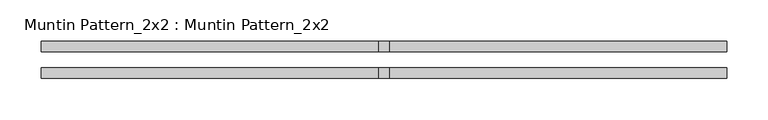
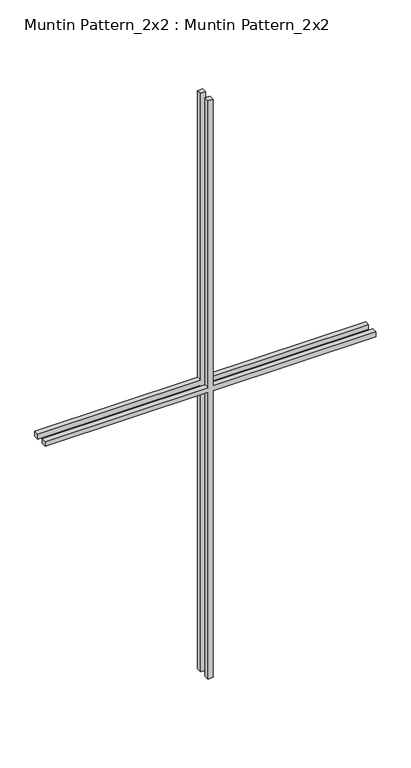
"""IFC4 building model written with IfcOpenShell, lengths in millimetres: proxy geometry, Muntin Pattern_2x2 : Muntin Pattern_2x2."""

from ifc_helpers import new_model, si_unit, frame, origin, place, context, project, spatial, polyline, outline, extrude, source, transform, mapped, element, save


def muntin_pattern_2x2_muntin_pattern_2x2_a6e57790(model_context):
    return source(origin(), model_context, "Body", "SweptSolid", [
        extrude(outline(polyline([(771.525, -6.35), (771.525, -414.3375), (758.825, -414.3375), (758.825, -6.35), (0.0, -6.35), (0.0, 6.35), (758.825, 6.35), (758.825, 414.3375), (771.525, 414.3375), (771.525, 6.35), (1530.35, 6.35), (1530.35, -6.35), (771.525, -6.35)])), frame((0.0, -22.225, 0.0), z_axis=(0.0, 1.0, 0.0), x_axis=(0.0, 0.0, 1.0)), (0.0, 0.0, 1.0), 12.7),
        extrude(outline(polyline([(771.525, -6.35), (771.525, -414.3375), (758.825, -414.3375), (758.825, -6.35), (0.0, -6.35), (0.0, 6.35), (758.825, 6.35), (758.825, 414.3375), (771.525, 414.3375), (771.525, 6.35), (1530.35, 6.35), (1530.35, -6.35), (771.525, -6.35)])), frame((0.0, 9.525, 0.0), z_axis=(0.0, 1.0, 0.0), x_axis=(0.0, 0.0, 1.0)), (0.0, 0.0, 1.0), 12.7),
    ])


if __name__ == "__main__":
    model = new_model("IFC4")
    model_context = context("Model", 3, world=origin())
    ifc_project = project(units=[si_unit("LENGTHUNIT", "METRE", prefix="MILLI")], contexts=[model_context])
    site = spatial("IfcSite", under=ifc_project)
    building = spatial("IfcBuilding", under=site)
    placement = place(None, origin())
    muntin_pattern_2x2_muntin_pattern_2x2_shape = muntin_pattern_2x2_muntin_pattern_2x2_a6e57790(model_context)
    element("IfcBuildingElementProxy", 1, Name="Muntin Pattern_2x2 : Muntin Pattern_2x2", ObjectType="Muntin Pattern_2x2 : Muntin Pattern_2x2", at=placement, inside=building, context=model_context, shape_type="MappedRepresentation", body=[
        mapped(muntin_pattern_2x2_muntin_pattern_2x2_shape, transform((0.0, 0.0, 0.0), x_axis=(1.0, 0.0, 0.0), y_axis=(0.0, 1.0, 0.0), z_axis=(0.0, 0.0, 1.0))),
    ])
    save(model, "model.ifc")

# Revit data of these elements
# Type "Muntin Pattern_2x2 : Muntin Pattern_2x2"
#   Width [instance default] = 4' - 0"
#   Thickness = 0' - 0 1/2"
#   Height [instance default] = 4' - 0"
#   Distance = 0' - 0 3/4"
#   Interior Material [instance default] = none
#   Exterior Material [instance default] = none
#   Default Elevation = 0
# Element 1 (IfcBuildingElementProxy, "Muntin Pattern_2x2 : Muntin Pattern_2x2")
#   Width = 2' - 8 5/8"
#   Height = 5' - 0 1/4"
#   Interior Material = Wood - Stained
#   Exterior Material = Clad - White
#   Materials on its faces: "Clad - White", "Wood - Stained"
# Materials
#   "Clad - White": class "Wood", colour RGB 242 242 238, transparency 0, Cost = 0
#   "Wood - Stained": class "Wood", colour RGB 224 178 126, transparency 0, Cost = 0
